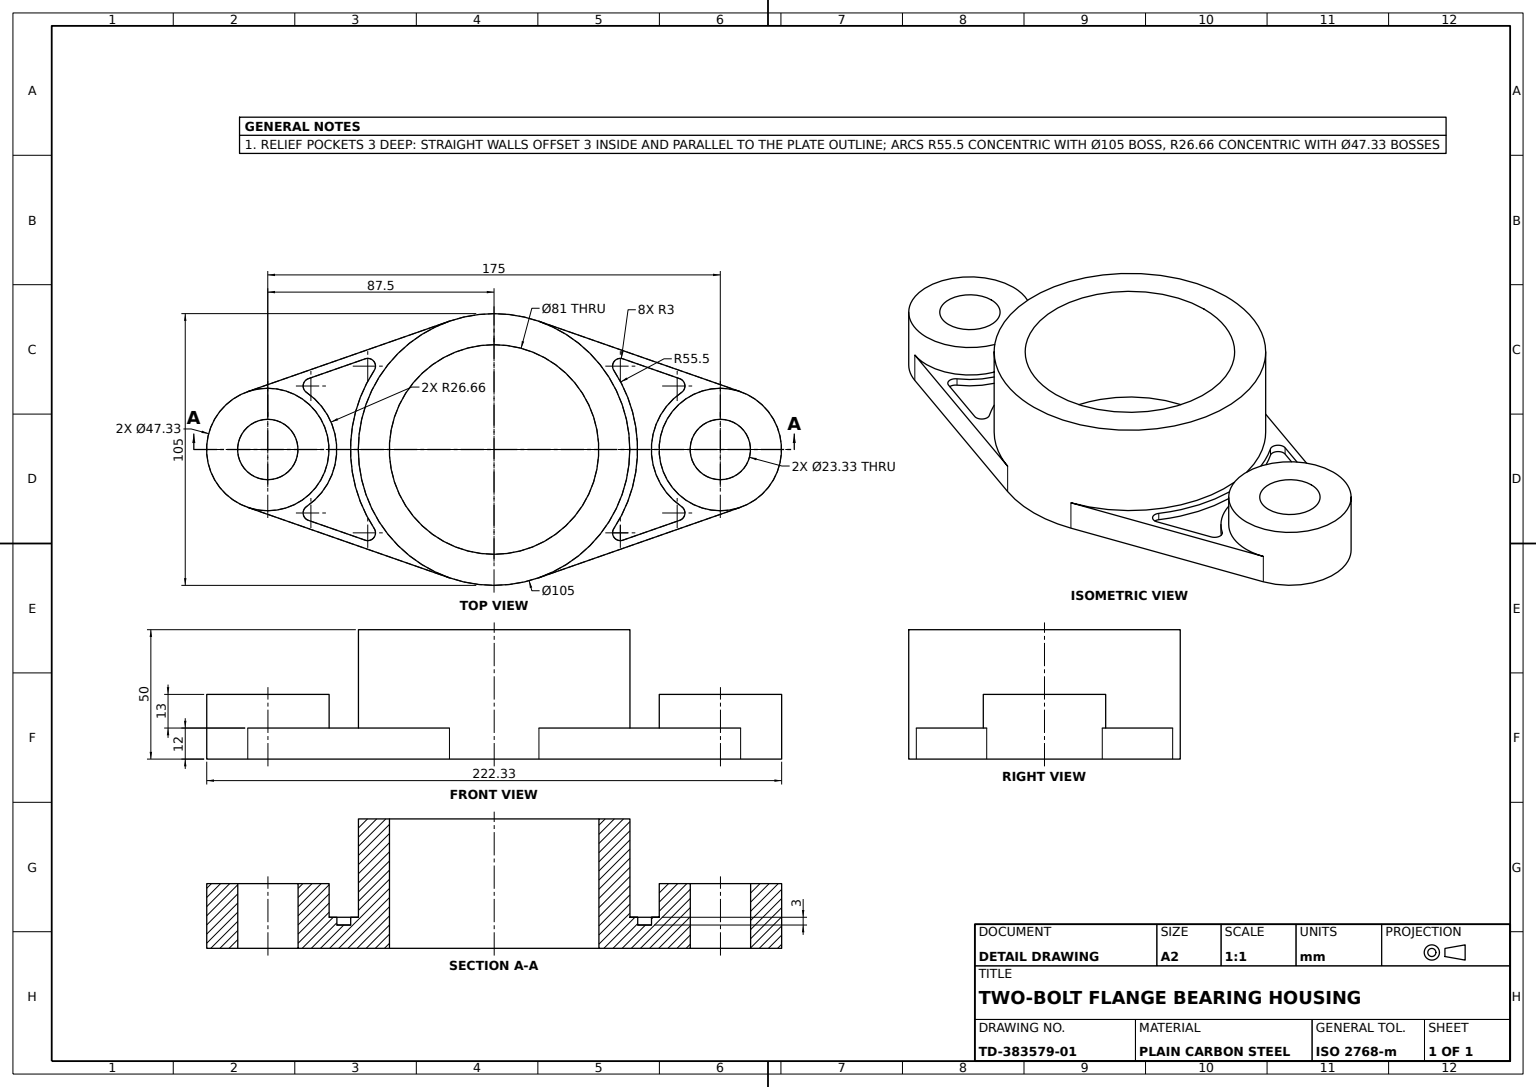
SolidWorks part; units mm, degrees
material "Plain Carbon Steel"
ref_plane "Front Plane" through (0, 0, 0) normal (0, 0, 1) x (1, 0, 0)
ref_plane "Top Plane" through (0, 0, 0) normal (0, 1, 0) x (1, 0, 0)
ref_plane "Right Plane" through (0, 0, 0) normal (1, 0, 0) x (0, 0, -1)
sketch "Flange Plate Sketch" plane through (0, 0, 0) normal (0, 1, 0) x (1, 0, 0)
  line L0 (-87.5, 0) -> (87.5, 0) construction
  line L3 (-17.301, 49.5674) -> (-95.2986, 22.3431)
  line L4 (17.301, 49.5674) -> (95.2986, 22.3431)
  line L5 (0, 0) -> (179.8704, 0) construction
  line L6 (-17.301, -49.5674) -> (-95.2986, -22.3431)
  line L7 (17.301, -49.5674) -> (95.2986, -22.3431)
  line L8 (0, 0) -> (0, 33.4298) construction
  arc A0 (-95.2986, 22.3431) -> (-95.2986, -22.3431) centre (-87.5, 0) ccw
  arc A1 (95.2986, -22.3431) -> (95.2986, 22.3431) centre (87.5, 0) ccw
  circle A3 centre (0, 0) radius 52.5
  circle A4 centre (-87.5, 0) radius 11.665
  circle A6 centre (87.5, 0) radius 11.665
  circle A8 centre (0, 0) radius 40.5
  point P3 (0, 0)
  dimension "D2" = 105
  dimension "D3" = 12
  dimension "D4" = 23.33
  dimension "D5" = 12
  dimension "D1" = 175
extrude "Flange Plate" add sketch "Flange Plate Sketch" along normal blind 12 contours A3 L3 A0 L6 A4 | A3 L7 A1 L4 A6 | A3 A8
sketch "Housing Boss Sketch" plane through (0, 12, 0) normal (0, 1, 0) x (1, 0, 0)
  circle A0 centre (0, 0) radius 40.5 construction
  circle A1 centre (0, 0) radius 40.5
  circle A2 centre (0, 0) radius 52.5
  dimension "D1" = 12
extrude "Bearing Housing Boss" add sketch "Housing Boss Sketch" along normal blind 38
sketch "Bolt Boss Sketch" plane through (0, 12, 0) normal (0, 1, 0) x (1, 0, 0)
  circle A0 centre (87.5, 0) radius 11.665 construction
  circle A1 centre (-87.5, 0) radius 11.665 construction
  circle A2 centre (87.5, 0) radius 11.665
  circle A3 centre (-87.5, 0) radius 11.665
  circle A4 centre (87.5, 0) radius 23.665
  circle A5 centre (-87.5, 0) radius 23.665
  dimension "D1" = 12
extrude "Bolt Bosses 2x" add sketch "Bolt Boss Sketch" along normal blind 13
sketch "Relief Pocket Sketch" plane through (0, 12, 0) normal (0, 1, 0) x (1, 0, 0)
  line L4 (78.3996, 25.064) -> (40.0101, 38.4635)
  line L5 (40.0101, -38.4635) -> (78.3996, -25.064)
  line L6 (71.8093, 27.3643) -> (49.826, 35.0373)
  line L7 (49.826, -35.0373) -> (71.8093, -27.3643)
  line L10 (-78.3996, -25.064) -> (-40.0101, -38.4635)
  line L11 (-40.0101, 38.4635) -> (-78.3996, 25.064)
  line L12 (-71.8093, -27.3643) -> (-49.826, -35.0373)
  line L13 (-49.826, 35.0373) -> (-71.8093, 27.3643)
  arc A4 (78.3996, 25.064) -> (78.3996, -25.064) centre (87.5, 0) ccw
  arc A5 (40.0101, -38.4635) -> (40.0101, 38.4635) centre (0, 0) ccw
  arc A6 (72.5075, 22.051) -> (72.5075, -22.051) centre (87.5, 0) ccw
  arc A7 (46.3329, -30.5534) -> (46.3329, 30.5534) centre (0, 0) ccw
  arc A8 (46.3329, -30.5534) -> (49.826, -35.0373) centre (48.8374, -32.2049) ccw
  arc A9 (72.5075, -22.051) -> (71.8093, -27.3643) centre (70.8207, -24.5319) cw
  arc A10 (-78.3996, -25.064) -> (-78.3996, 25.064) centre (-87.5, 0) ccw
  arc A11 (-40.0101, 38.4635) -> (-40.0101, -38.4635) centre (0, 0) ccw
  arc A12 (-72.5075, -22.051) -> (-72.5075, 22.051) centre (-87.5, 0) ccw
  arc A13 (-46.3329, 30.5534) -> (-46.3329, -30.5534) centre (0, 0) ccw
  arc A14 (72.5075, 22.051) -> (71.8093, 27.3643) centre (70.8207, 24.5319) ccw
  arc A15 (49.826, 35.0373) -> (46.3329, 30.5534) centre (48.8374, 32.2049) ccw
  arc A16 (-72.5075, -22.051) -> (-71.8093, -27.3643) centre (-70.8207, -24.5319) ccw
  arc A17 (-49.826, -35.0373) -> (-46.3329, -30.5534) centre (-48.8374, -32.2049) ccw
  arc A18 (-46.3329, 30.5534) -> (-49.826, 35.0373) centre (-48.8374, 32.2049) ccw
  arc A19 (-72.5075, 22.051) -> (-71.8093, 27.3643) centre (-70.8207, 24.5319) cw
  dimension "D3" = 3
  dimension "D1" = 3
  dimension "D2" = 3
extrude "Flange Relief Pockets" cut sketch "Relief Pocket Sketch" against normal blind 3
